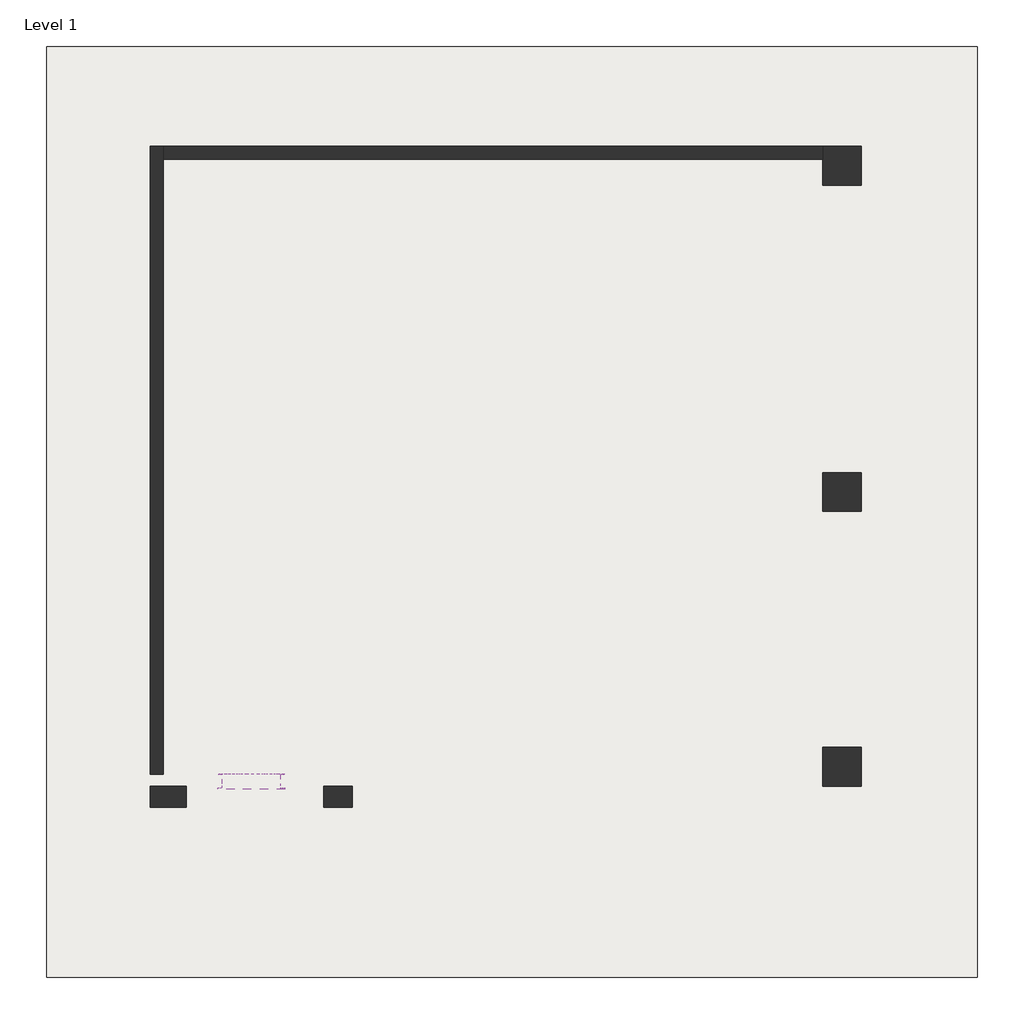
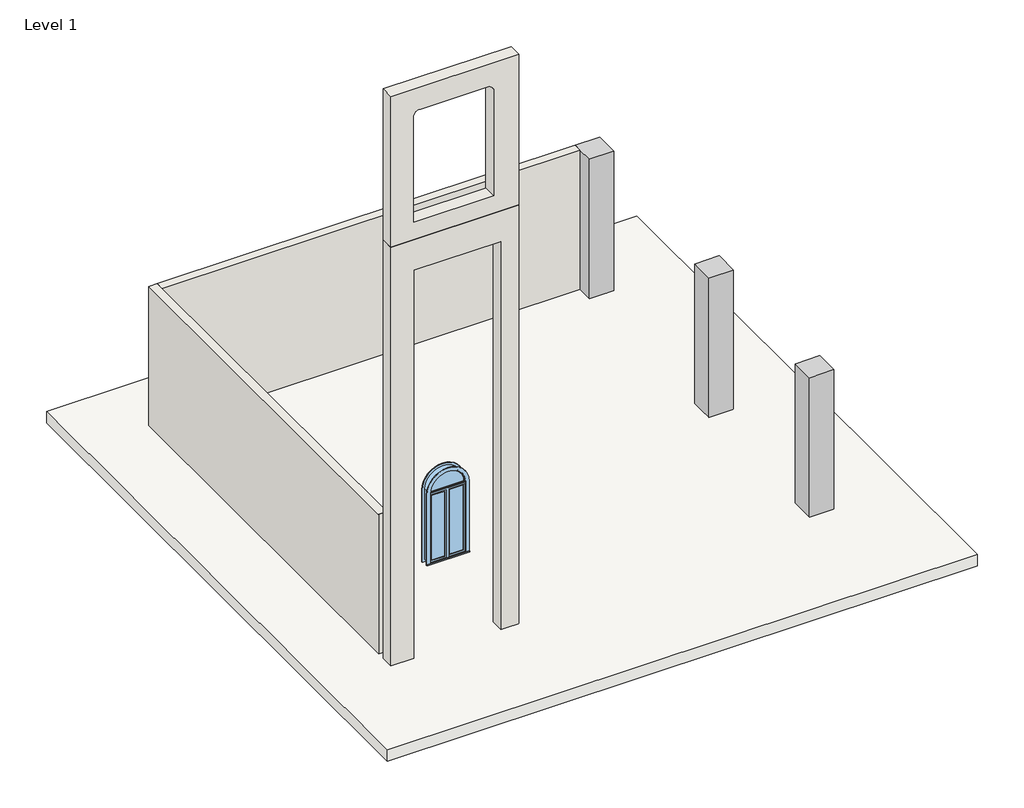
# One storey: 3 columns, 3 walls, 1 slab, 1 window.
"""IFC4 building model written with IfcOpenShell, lengths in millimetres."""

from ifc_helpers import new_model, si_unit, frame, origin, origin_with_axes, place, context, project, spatial, polyline, outline, extrude, faceted_brep, transform, mapped, element, save
from components import walls_1_walls_1_151b54a8, window_4e95f2a8

model = new_model("IFC4")

# Units and contexts
model_context = context("Model", 3, world=origin())
ifc_project = project(units=[si_unit("LENGTHUNIT", "METRE", prefix="MILLI")], contexts=[model_context])

# Site, building, storey
site = spatial("IfcSite", under=ifc_project)
building = spatial("IfcBuilding", under=site)
storey = spatial("IfcBuildingStorey", under=building, Name="Level 1", Elevation=0.0)

# Columns
placement = place(None, origin())
element("IfcColumn", 1, ObjectType="Rectangular Column : 24\" x 24\"", at=placement, inside=storey, context=model_context, shape_type="Brep", body=[
    faceted_brep([(2149.5001186, 882.3610824, 3657.6), (1539.9001186, 882.3610824, 3657.6), (1539.9001186, 272.7610824, 3657.6), (2149.5001186, 272.7610824, 3657.6), (2149.5001186, 475.9610824, 3657.6), (2149.5001186, 882.3610824, 0.0), (2149.5001186, 272.7610824, 0.0), (1539.9001186, 272.7610824, 0.0), (1539.9001186, 882.3610824, 0.0)], [[[0, 1, 2, 3, 4]], [[5, 6, 7, 8]], [[1, 0, 5, 8]], [[2, 1, 8, 7]], [[3, 2, 7, 6]], [[0, 4, 3, 6, 5]]]),
])
element("IfcColumn", 2, ObjectType="Rectangular Column : 24\" x 24\"", at=placement, inside=storey, context=model_context, shape_type="SweptSolid", body=[
    extrude(outline(polyline([(2149.5001186, 5200.3610824), (2149.5001186, 4590.7610824), (1539.9001186, 4590.7610824), (1539.9001186, 5200.3610824), (2149.5001186, 5200.3610824)])), origin_with_axes(), (0.0, 0.0, 1.0), 3657.6),
])
element("IfcColumn", 3, ObjectType="Rectangular Column : 24\" x 24\"", at=placement, inside=storey, context=model_context, shape_type="Brep", body=[
    faceted_brep([(2149.5001186, 10331.1610824, 3657.6), (1539.9001186, 10331.1610824, 3657.6), (1539.9001186, 10127.9610824, 3657.6), (1539.9001186, 9721.5610824, 3657.6), (2149.5001186, 9721.5610824, 3657.6), (2149.5001186, 10127.9610824, 3657.6), (2149.5001186, 10331.1610824, 0.0), (2149.5001186, 9721.5610824, 0.0), (1539.9001186, 9721.5610824, 0.0), (1539.9001186, 10127.9610824, 0.0), (1539.9001186, 10331.1610824, 0.0)], [[[0, 1, 2, 3, 4, 5]], [[6, 7, 8, 9, 10]], [[1, 0, 6, 10]], [[3, 2, 1, 10, 9, 8]], [[4, 3, 8, 7]], [[0, 5, 4, 7, 6]]]),
])

# Slab
element("IfcSlab", 4, ObjectType="Generic - 12\"", at=placement, inside=storey, context=model_context, shape_type="SweptSolid", body=[
    extrude(outline(polyline([(3972.606595, 11898.2733643), (3972.606595, -2732.1266357), (-10657.793405, -2732.1266357), (-10657.793405, 11898.2733643), (3972.606595, 11898.2733643)])), frame((0.0, 0.0, -304.8), z_axis=(0.0, 0.0, 1.0), x_axis=(1.0, 0.0, 0.0)), (0.0, 0.0, 1.0), 304.8),
])

# Walls
element("IfcWall", 5, ObjectType="Generic - 8\"", at=placement, inside=storey, context=model_context, shape_type="Brep", body=[
    faceted_brep([(-8823.2998814, 463.2610824, 0.0), (-8823.2998814, 10127.9610824, 0.0), (-8823.2998814, 10331.1610824, 0.0), (-8823.2998814, 10331.1610824, 3657.6), (-8823.2998814, 10127.9610824, 3657.6), (-8823.2998814, 475.9610824, 3657.6), (-8823.2998814, 463.2610824, 3657.6), (-9026.4998814, 463.2610824, 0.0), (-9026.4998814, 463.2610824, 3657.6), (-9026.4998814, 475.9610824, 3657.6), (-9026.4998814, 10331.1610824, 3657.6), (-9026.4998814, 10331.1610824, 0.0)], [[[0, 1, 2, 3, 4, 5, 6]], [[7, 8, 9, 10, 11]], [[2, 1, 0, 7, 11]], [[0, 6, 8, 7]], [[6, 5, 9, 8]], [[5, 4, 3, 10, 9]], [[3, 2, 11, 10]]]),
])
element("IfcWall", 6, ObjectType="Generic - 8\"", at=placement, inside=storey, context=model_context, shape_type="SweptSolid", body=[
    extrude(outline(polyline([(1539.9001186, 10127.9610824), (-8823.2998814, 10127.9610824), (-8823.2998814, 10331.1610824), (1539.9001186, 10331.1610824), (1539.9001186, 10127.9610824)])), origin_with_axes(), (0.0, 0.0, 1.0), 3657.6),
])
walls_1_walls_1_shape = walls_1_walls_1_151b54a8(model_context)
element("IfcWall", 7, ObjectType="Walls 1 : Walls 1", at=placement, inside=storey, context=model_context, shape_type="MappedRepresentation", body=[
    mapped(walls_1_walls_1_shape, transform((0.0, 0.0, 0.0), x_axis=(1.0, 0.0, 0.0), y_axis=(0.0, 1.0, 0.0), z_axis=(0.0, 0.0, 1.0))),
])

# Window
window_shape = window_4e95f2a8(model_context)
element("IfcWindow", 8, ObjectType="36\" x 72\"", at=placement, inside=storey, context=model_context, shape_type="MappedRepresentation", body=[
    mapped(window_shape, transform((-7430.9977233, 348.9610824, 1783.024), x_axis=(-1.0, 0.0, 0.0), y_axis=(0.0, -1.0, 0.0), z_axis=(0.0, 0.0, 1.0))),
])

save(model, "model.ifc")

# Revit data of these elements
# Type "Rectangular Column : 24\" x 24\""
#   Assembly Code = "B1010200"
#   Depth = 2' - 0"
#   Offset Base = 0' - 0"
#   Offset Top = 0' - 0"
#   Width = 2' - 0"
#   Material = none
# Type "Generic - 12\""
#   Assembly Code = "B1010"
#   Function = 0
#   Layers, outside or top first: 1' - 0" no material (function 1)
# Type "Generic - 8\""
#   Assembly Code = "B2010"
#   Layers, outside or top first: 0' - 8" no material (function 1)
# Type "36\" x 72\""
#   Type Mark = "10"
#   Construction Type Id = "SGL"
#   Assembly Code = "B2020100"
#   Analytic Construction = "Large single-glazed windows"
#   Visual Light Transmittance = 0.9
#   Solar Heat Gain Coefficient = 0.86
#   Heat Transfer Coefficient (U) = 0.979472 BTU/(h·ft²·°F)
#   Height = 6' - 0"
#   Default Sill Height = 1' - 0"
#   Trim Projection - Ext. = 0' - 0 1/2"
#   Trim Projection - Int. = 0' - 0 3/4"
#   Trim Width - Exterior = 0' - 3 1/2"
#   Trim Width - Interior = 0' - 3 1/2"
#   Width = 3' - 0"
#   Window Inset = 0' - 0 3/4"
#   Define Thermal Properties by = 1
#   Glass Pane Material = Glass
#   Sash Material = Sash
#   Trim Exterior Material = Trim
#   Trim Interior Material = Trim
#   Wall Closure = (empty or 0)
# Elements 1, 2, 3 (IfcColumn, "Rectangular Column : 24\" x 24\"")
#   Phase Created = New Construction
#   Materials on its faces: "Default Wall"
# Element 4 (IfcSlab, "Generic - 12\"")
#   Height Offset From Level = 0' - 0"
#   Phase Created = New Construction
#   Materials on its faces: "Default Floor"
# Elements 5, 6 (IfcWall, "Generic - 8\"")
#   Top Offset = 0' - 0"
#   Base Offset = 0' - 0"
#   Unconnected Height = 12' - 0"
#   wall height = 12' - 0"
#   Phase Created = New Construction
#   Base Constraint = Level 1
#   Materials on its faces: "Default Wall"
# Element 7 (IfcWall, "Walls 1 : Walls 1")
#   Phase Created = New Construction
#   Materials on its faces: "Default Wall"
# Element 8 (IfcWindow, "36\" x 72\"")
#   Mark = "2"
#   Phase Created = New Construction
#   Materials on its faces: "Sash", "Trim", "Glass"
# Materials
#   "Glass": class "Glass", colour RGB 0 128 192, transparency 0.75, Description = "Soda Lime Glass", Cost = 0
#   "Sash": class "Wood", colour RGB 224 178 126, transparency 0
#   "Trim": class "Wood", colour RGB 224 178 126, transparency 0
#   "Default Wall": colour RGB 128 128 128, transparency 0
#   "Default Floor": colour RGB 128 128 128, transparency 0
